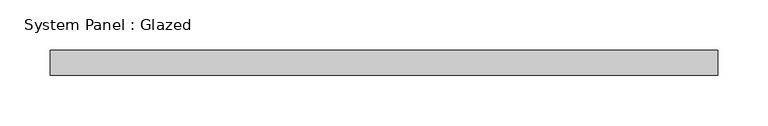
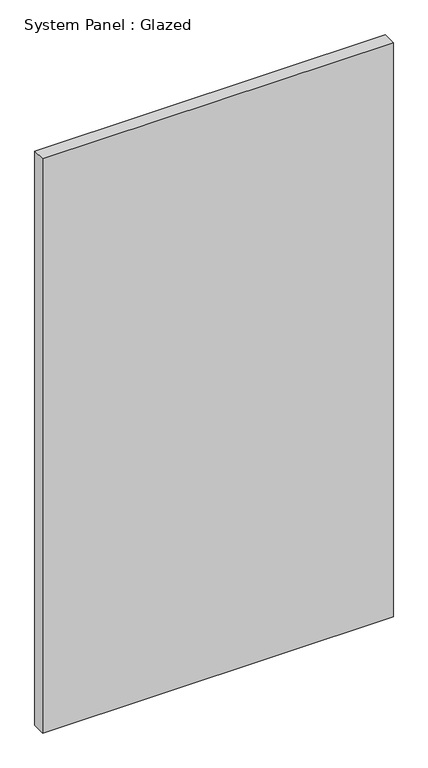
"""IFC4 building model written with IfcOpenShell, lengths in millimetres: plate geometry, System Panel : Glazed."""

from ifc_helpers import new_model, si_unit, origin, origin_with_axes, place, context, project, spatial, polyline, outline, extrude, source, transform, mapped, element, save


def system_panel_glazed_cc8aff5a(model_context):
    return source(origin(), model_context, "Body", "SweptSolid", [
        extrude(outline(polyline([(333.9348534, 19.05), (-333.9348534, 19.05), (-333.9348534, 44.45), (333.9348534, 44.45), (333.9348534, 19.05)])), origin_with_axes(), (0.0, 0.0, 1.0), 1155.7),
    ])


if __name__ == "__main__":
    model = new_model("IFC4")
    model_context = context("Model", 3, world=origin())
    ifc_project = project(units=[si_unit("LENGTHUNIT", "METRE", prefix="MILLI")], contexts=[model_context])
    site = spatial("IfcSite", under=ifc_project)
    building = spatial("IfcBuilding", under=site)
    placement = place(None, origin())
    system_panel_glazed_shape = system_panel_glazed_cc8aff5a(model_context)
    element("IfcPlate", 1, ObjectType="System Panel : Glazed", at=placement, inside=building, context=model_context, shape_type="MappedRepresentation", body=[
        mapped(system_panel_glazed_shape, transform((0.0, 0.0, 0.0), x_axis=(1.0, 0.0, 0.0), y_axis=(0.0, 1.0, 0.0), z_axis=(0.0, 0.0, 1.0))),
    ])
    save(model, "model.ifc")

# Revit data of these elements
# Type "System Panel : Glazed"
#   Construction Type Id = "GSP4R"
#   Analytic Construction = "1/8 in Pilkington single glazing"
#   Visual Light Transmittance = 0.9
#   Solar Heat Gain Coefficient = 0.86
#   Heat Transfer Coefficient (U) = 1.18115 BTU/(h·ft²·°F)
# Element 1 (IfcPlate, "System Panel : Glazed")
#   Materials on its faces: "Glass"
# Materials
#   "Glass": class "Glass", colour RGB 0 128 192, transparency 0.75, Description = "Soda Lime Glass", Cost = 0
